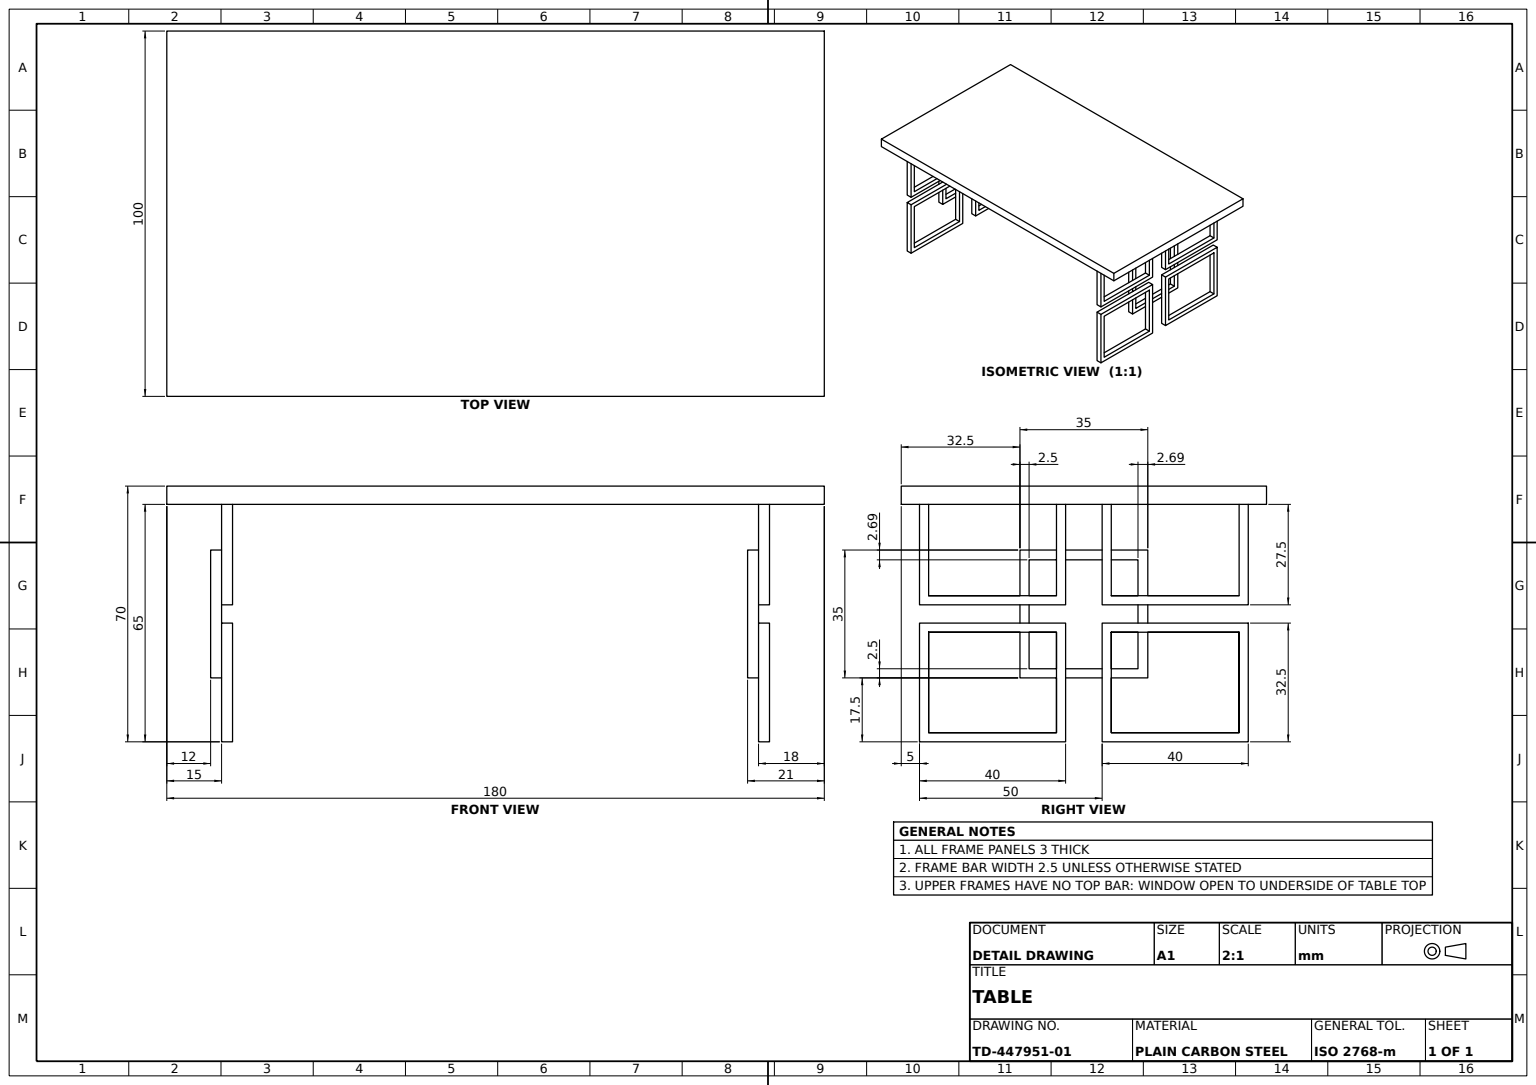
from build123d import *

# Parameters (mm, degrees)
FRONT_FRAME_PANEL_SKETCH_W      = 40
FRONT_FRAME_PANEL_SKETCH_H      = 32.5
FRONT_FRAME_PANEL_40X32_5_DEPTH = 3
FRONT_FRAME_SIDE_SKETCH_W       = 40
FRONT_FRAME_SIDE_SKETCH_H       = 32.5
FRONT_FRAME_SIDE_DEPTH          = 3
FRONT_FRAME_OUTER_SKETCH_W      = 40
FRONT_FRAME_OUTER_SKETCH_H      = 32.5
FRONT_FRAME_OUTER_DEPTH         = 3
FRONT_FRAME_OUTER_2_DEPTH       = 3
FRAME_WINDOW_CUT_SKETCH_W       = 35
FRAME_WINDOW_CUT_SKETCH_H       = 27.5
FRAME_WINDOW_CUT_DEPTH          = 3
FRONT_SQUARE_FRAME_SKETCH_W     = 35
FRONT_SQUARE_FRAME_SKETCH_H     = 35
FRONT_SQUARE_FRAME_SKETCH_W_2   = 29.813797942
FRONT_SQUARE_FRAME_SKETCH_H_2   = 29.813797942
FRONT_SQUARE_FRAME_35X35_DEPTH  = 3
REAR_FRAME_A_SKETCH_W           = 40
REAR_FRAME_A_SKETCH_H           = 32.5
REAR_FRAME_A_SKETCH_W_2         = 35
REAR_FRAME_A_SKETCH_H_2         = 27.5
REAR_FRAME_A_DEPTH              = 3
REAR_FRAME_B_SKETCH_W           = 40
REAR_FRAME_B_SKETCH_H           = 32.5
REAR_FRAME_B_SKETCH_W_2         = 35
REAR_FRAME_B_SKETCH_H_2         = 27.5
REAR_FRAME_B_DEPTH              = 3
REAR_FRAME_C_SKETCH_W           = 40
REAR_FRAME_C_SKETCH_H           = 32.5
REAR_FRAME_C_SKETCH_W_2         = 35
REAR_FRAME_C_SKETCH_H_2         = 27.5
REAR_FRAME_C_DEPTH              = 3
REAR_FRAME_D_SKETCH_W           = 40
REAR_FRAME_D_SKETCH_H           = 32.5
REAR_FRAME_D_SKETCH_W_2         = 35
REAR_FRAME_D_SKETCH_H_2         = 27.5
REAR_FRAME_D_DEPTH              = 3
REAR_SQUARE_FRAME_SKETCH_W      = 35
REAR_SQUARE_FRAME_SKETCH_H      = 35
REAR_SQUARE_FRAME_SKETCH_W_2    = 29.813797942
REAR_SQUARE_FRAME_SKETCH_H_2    = 29.813797942
REAR_SQUARE_FRAME_DEPTH         = 3
TABLE_TOP_162X100X5_DEPTH       = 5


with BuildPart() as part:
    # Front Frame Panel Sketch → Front Frame Panel 40x32.5 (new body)
    with BuildSketch(Plane.XY):
        with Locations((20, 16.25)):
            Rectangle(FRONT_FRAME_PANEL_SKETCH_W, FRONT_FRAME_PANEL_SKETCH_H)
    extrude(amount=FRONT_FRAME_PANEL_40X32_5_DEPTH)


with BuildPart() as body_2:
    # Front Frame Side Sketch → Front Frame Side (new body)
    with BuildSketch(Plane.XY.offset(3)):
        with Locations((70, 16.25)):
            Rectangle(FRONT_FRAME_SIDE_SKETCH_W, FRONT_FRAME_SIDE_SKETCH_H)
    extrude(amount=-FRONT_FRAME_SIDE_DEPTH)


with BuildPart() as body_3:
    # Front Frame Outer Sketch → Front Frame Outer (new body)
    with BuildSketch(Plane.XY.offset(3)):
        with Locations((20, 53.75)):
            Rectangle(FRONT_FRAME_OUTER_SKETCH_W, FRONT_FRAME_OUTER_SKETCH_H)
    extrude(amount=-FRONT_FRAME_OUTER_DEPTH)


with BuildPart() as body_4:
    # Front Frame Outer Sketch → Front Frame Outer 2 (new body)
    with BuildSketch(Plane.XY.offset(3)):
        with Locations((70, 53.75)):
            Rectangle(FRONT_FRAME_OUTER_SKETCH_W, FRONT_FRAME_OUTER_SKETCH_H)
    extrude(amount=-FRONT_FRAME_OUTER_2_DEPTH)


with BuildPart() as frame_window_cut_tool:
    # Frame Window Cut Sketch → Frame Window Cut (new body)
    with BuildSketch(Plane.XY.offset(3)):
        with Locations((20, 16.25)):
            Rectangle(FRAME_WINDOW_CUT_SKETCH_W, FRAME_WINDOW_CUT_SKETCH_H)
        with Locations((70, 16.25)):
            Rectangle(FRAME_WINDOW_CUT_SKETCH_W, FRAME_WINDOW_CUT_SKETCH_H)
        with Locations((20, 53.75)):
            Rectangle(FRAME_WINDOW_CUT_SKETCH_W, FRAME_WINDOW_CUT_SKETCH_H)
        with Locations((70, 53.75)):
            Rectangle(FRAME_WINDOW_CUT_SKETCH_W, FRAME_WINDOW_CUT_SKETCH_H)
    extrude(amount=-FRAME_WINDOW_CUT_DEPTH)


with BuildPart() as part_1:
    add(part.part)

    # Frame Window Cut: cut by frame_window_cut_tool
    add(frame_window_cut_tool.part, mode=Mode.SUBTRACT)



with BuildPart() as body_2_1:
    add(body_2.part)

    # Frame Window Cut: cut by frame_window_cut_tool
    add(frame_window_cut_tool.part, mode=Mode.SUBTRACT)


with BuildPart() as body_3_1:
    add(body_3.part)

    # Frame Window Cut: cut by frame_window_cut_tool
    add(frame_window_cut_tool.part, mode=Mode.SUBTRACT)


with BuildPart() as body_4_1:
    add(body_4.part)

    # Frame Window Cut: cut by frame_window_cut_tool
    add(frame_window_cut_tool.part, mode=Mode.SUBTRACT)


with BuildPart() as part_2:
    add(part_1.part)

    add(body_2_1.part)  # Front Square Frame 35x35 merges body 2

    add(body_3_1.part)  # Front Square Frame 35x35 merges body 3

    add(body_4_1.part)  # Front Square Frame 35x35 merges body 4
    # Front Square Frame Sketch → Front Square Frame 35x35 (add)
    with BuildSketch(Plane.XY.offset(3)):
        with Locations((45, 35)):
            Rectangle(FRONT_SQUARE_FRAME_SKETCH_W, FRONT_SQUARE_FRAME_SKETCH_H)
        with Locations((45.093101029, 34.906898971)):
            Rectangle(FRONT_SQUARE_FRAME_SKETCH_W_2, FRONT_SQUARE_FRAME_SKETCH_H_2, mode=Mode.SUBTRACT)
    extrude(amount=FRONT_SQUARE_FRAME_35X35_DEPTH)



with BuildPart() as body_2_2:
    # Rear Frame A Sketch → Rear Frame A (new body)
    with BuildSketch(Plane.XY.offset(-147)):
        with Locations((70, 16.25)):
            Rectangle(REAR_FRAME_A_SKETCH_W, REAR_FRAME_A_SKETCH_H)
        with Locations((70, 16.25)):
            Rectangle(REAR_FRAME_A_SKETCH_W_2, REAR_FRAME_A_SKETCH_H_2, mode=Mode.SUBTRACT)
    extrude(amount=REAR_FRAME_A_DEPTH)



with BuildPart() as body_3_2:
    # Rear Frame B Sketch → Rear Frame B (new body)
    with BuildSketch(Plane.XY.offset(-147)):
        with Locations((20, 16.25)):
            Rectangle(REAR_FRAME_B_SKETCH_W, REAR_FRAME_B_SKETCH_H)
        with Locations((20, 16.25)):
            Rectangle(REAR_FRAME_B_SKETCH_W_2, REAR_FRAME_B_SKETCH_H_2, mode=Mode.SUBTRACT)
    extrude(amount=REAR_FRAME_B_DEPTH)


with BuildPart() as body_4_2:
    # Rear Frame C Sketch → Rear Frame C (new body)
    with BuildSketch(Plane.XY.offset(-147)):
        with Locations((20, 53.75)):
            Rectangle(REAR_FRAME_C_SKETCH_W, REAR_FRAME_C_SKETCH_H)
        with Locations((20, 53.75)):
            Rectangle(REAR_FRAME_C_SKETCH_W_2, REAR_FRAME_C_SKETCH_H_2, mode=Mode.SUBTRACT)
    extrude(amount=REAR_FRAME_C_DEPTH)


with BuildPart() as body_5:
    # Rear Frame D Sketch → Rear Frame D (new body)
    with BuildSketch(Plane.XY.offset(-147)):
        with Locations((70, 53.75)):
            Rectangle(REAR_FRAME_D_SKETCH_W, REAR_FRAME_D_SKETCH_H)
        with Locations((70, 53.75)):
            Rectangle(REAR_FRAME_D_SKETCH_W_2, REAR_FRAME_D_SKETCH_H_2, mode=Mode.SUBTRACT)
    extrude(amount=REAR_FRAME_D_DEPTH)


with BuildPart() as body_2_2_1:
    add(body_2_2.part)

    add(body_3_2.part)  # Rear Square Frame merges body 3 2

    add(body_4_2.part)  # Rear Square Frame merges body 4 2

    add(body_5.part)  # Rear Square Frame merges body 5
    # Rear Square Frame Sketch → Rear Square Frame (add)
    with BuildSketch(Plane.XY.offset(-144)):
        with Locations((45, 35)):
            Rectangle(REAR_SQUARE_FRAME_SKETCH_W, REAR_SQUARE_FRAME_SKETCH_H)
        with Locations((45.093101029, 34.906898971)):
            Rectangle(REAR_SQUARE_FRAME_SKETCH_W_2, REAR_SQUARE_FRAME_SKETCH_H_2, mode=Mode.SUBTRACT)
    extrude(amount=REAR_SQUARE_FRAME_DEPTH)


with BuildPart() as part_3:
    add(part_2.part)

    add(body_2_2_1.part)  # Table Top 162x100x5 merges body 2 2
    # Table Top Sketch → Table Top 162x100x5 (add)
    with BuildSketch(Plane(origin=(0, 70, 0), x_dir=(1, 0, 0), z_dir=(0, 1, 0))):
        Polygon((-5, 0), (-5, 162), (95, 162), (95, -18), (-5, -18), align=None)
    extrude(amount=-TABLE_TOP_162X100X5_DEPTH)


solid = part_3.part
